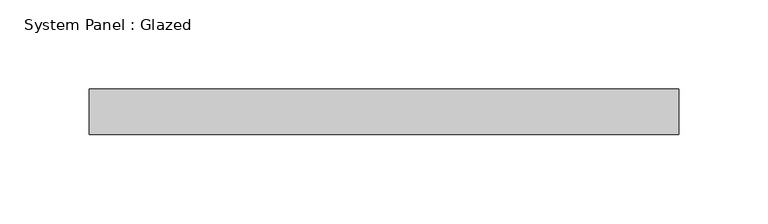
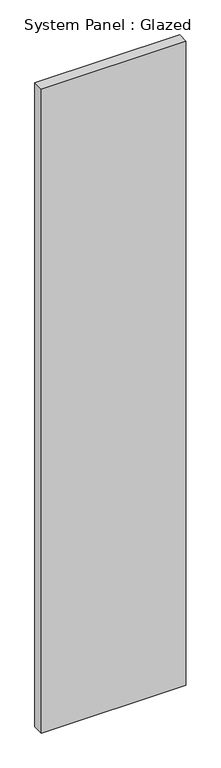
"""IFC4 building model written with IfcOpenShell, lengths in millimetres: plate geometry, System Panel : Glazed."""

from ifc_helpers import new_model, si_unit, origin, origin_with_axes, place, context, project, spatial, polyline, outline, extrude, source, transform, mapped, element, save


def system_panel_glazed_52ab50c3(model_context):
    return source(origin(), model_context, "Body", "SweptSolid", [
        extrude(outline(polyline([(165.1, 19.05), (-165.1, 19.05), (-165.1, 44.45), (165.1, 44.45), (165.1, 19.05)])), origin_with_axes(), (0.0, 0.0, 1.0), 1554.1349385),
    ])


if __name__ == "__main__":
    model = new_model("IFC4")
    model_context = context("Model", 3, world=origin())
    ifc_project = project(units=[si_unit("LENGTHUNIT", "METRE", prefix="MILLI")], contexts=[model_context])
    site = spatial("IfcSite", under=ifc_project)
    building = spatial("IfcBuilding", under=site)
    placement = place(None, origin())
    system_panel_glazed_shape = system_panel_glazed_52ab50c3(model_context)
    element("IfcPlate", 1, ObjectType="System Panel : Glazed", at=placement, inside=building, context=model_context, shape_type="MappedRepresentation", body=[
        mapped(system_panel_glazed_shape, transform((0.0, 0.0, 0.0), x_axis=(1.0, 0.0, 0.0), y_axis=(0.0, 1.0, 0.0), z_axis=(0.0, 0.0, 1.0))),
    ])
    save(model, "model.ifc")

# Revit data of these elements
# Type "System Panel : Glazed"
#   Construction Type Id = "GSP4R"
#   Analytic Construction = "1/8 in Pilkington single glazing"
#   Visual Light Transmittance = 0.9
#   Solar Heat Gain Coefficient = 0.86
#   Heat Transfer Coefficient (U) = 1.18115 BTU/(h·ft²·°F)
#   Define Thermal Properties by = 1
# Element 1 (IfcPlate, "System Panel : Glazed")
#   Materials on its faces: "Glass"
# Materials
#   "Glass": class "Glass", colour RGB 0 128 192, transparency 0.75, Description = "Soda Lime Glass", Cost = 0
